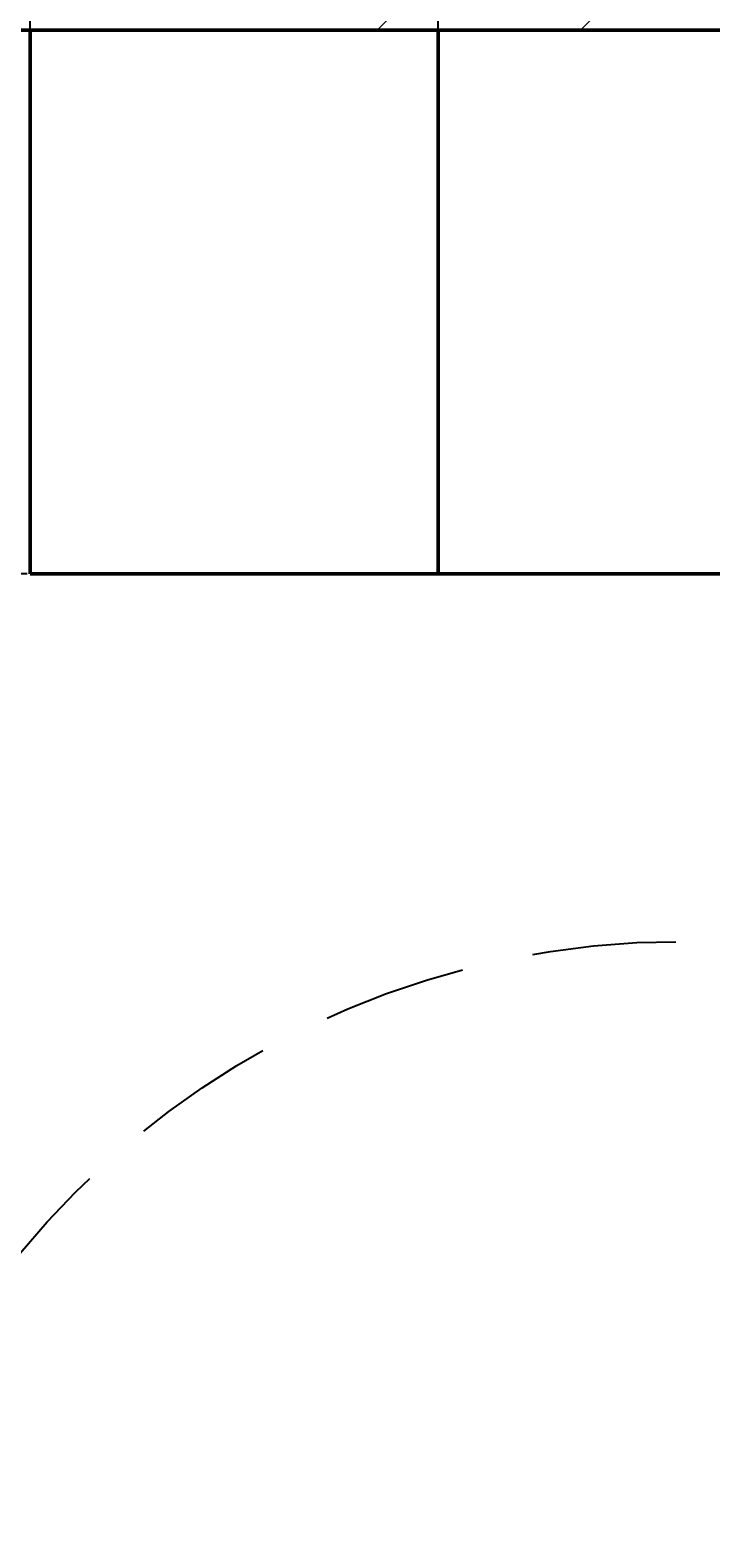
# Model space of a CAD drawing. Units: inches. Extents: x 2812 to 3051, y 1398 to 1659.
# Tile 54 of 65: x 2896 to 2911, y 1605 to 1638. Entities that reach past the tile are written whole.
import ezdxf

# ---------------------------------------------------------------- set-up
doc = ezdxf.new("R2010")
doc.units = ezdxf.units.IN
doc.linetypes.add('HIDDEN2', pattern=[4.7625, 3.175, -1.5875])
for name, color, linetype, lineweight in [('A-ANNO-DIMS', 2, 'Continuous', 18), ('S-CONC', 7, 'Continuous', 50), ('S-CONC-HIDN', 8, 'HIDDEN2', 25), ('S-CONC-PATT', 8, 'Continuous', 18)]:
    doc.layers.add(name, color=color, linetype=linetype, lineweight=lineweight)
doc.styles.get("Standard").update_dxf_attribs({"font": 'arial.ttf'})
doc.dimstyles.get("Standard").update_dxf_attribs({"dimtxt": 0.18, "dimasz": 0.18, "dimexe": 0.18, "dimexo": 0.0625, "dimgap": 0.09, "dimtad": 0, "dimtih": 1, "dimtoh": 1, "dimdec": 4, "dimzin": 0, "dimdsep": 46, "dimtxsty": 'Standard', "dimcen": 0.09, "dimadec": 0, "dimazin": 0, "dimtfac": 1, "dimtdec": 4, "dimtofl": 0, "dimtmove": 0, "dimatfit": 3, "dimfxl": 1, "dimtolj": 1, "dimtzin": 0, "dimarcsym": 0})

# ---------------------------------------------------------------- blocks, each defined once
blk = doc.blocks.new('*D18')
at = {"layer": 'A-ANNO-DIMS', "color": 0, "lineweight": -2, "transparency": 16777216}
for p, q in [((2896.385, 1625.882), (2896.385, 1659.35)), ((2905.385, 1625.882), (2905.385, 1659.35)), ((2896.565, 1659.17), (2900.736, 1659.17)), ((2905.205, 1659.17), (2901.034, 1659.17))]:
    blk.add_line(p, q, dxfattribs=at)
at = {"layer": 'A-ANNO-DIMS', "color": 0, "transparency": 16777216}
for points in [[(2896.565, 1659.2), (2896.565, 1659.14), (2896.385, 1659.17)], [(2905.205, 1659.2), (2905.205, 1659.14), (2905.385, 1659.17)]]:
    blk.add_solid(points, dxfattribs=at)
at = {"layer": 'Defpoints', "color": 0, "transparency": 16777216}
for p in [(2905.385, 1659.17), (2896.385, 1625.82), (2905.385, 1625.82)]:
    blk.add_point(p, dxfattribs=at)
at = {"layer": 'A-ANNO-DIMS', "color": 0, "transparency": 16777216, "insert": (2900.885, 1659.17), "char_height": 0.18, "attachment_point": 5}
blk.add_mtext('\\A1;9', dxfattribs=at)
blk = doc.blocks.new('*D19')
at = {"layer": 'A-ANNO-DIMS', "color": 0, "lineweight": -2, "transparency": 16777216}
for p, q in [((2905.385, 1625.882), (2905.385, 1659.35)), ((2941.385, 1625.882), (2941.385, 1659.35)), ((2905.565, 1659.17), (2923.166, 1659.17)), ((2941.205, 1659.17), (2923.604, 1659.17))]:
    blk.add_line(p, q, dxfattribs=at)
at = {"layer": 'A-ANNO-DIMS', "color": 0, "transparency": 16777216}
for points in [[(2905.565, 1659.2), (2905.565, 1659.14), (2905.385, 1659.17)], [(2941.205, 1659.2), (2941.205, 1659.14), (2941.385, 1659.17)]]:
    blk.add_solid(points, dxfattribs=at)
at = {"layer": 'Defpoints', "color": 0, "transparency": 16777216}
for p in [(2941.385, 1659.17), (2905.385, 1625.82), (2941.385, 1625.82)]:
    blk.add_point(p, dxfattribs=at)
at = {"layer": 'A-ANNO-DIMS', "color": 0, "transparency": 16777216, "insert": (2923.385, 1659.17), "char_height": 0.18, "attachment_point": 5}
blk.add_mtext('\\A1;36', dxfattribs=at)
blk = doc.blocks.new('*D38')
at = {"layer": 'A-ANNO-DIMS', "color": 0, "lineweight": -2, "transparency": 16777216}
for p, q in [((2896.322, 1625.82), (2811.806, 1625.82)), ((2811.986, 1625.64), (2811.986, 1612.5)), ((2811.986, 1599), (2811.986, 1612.14)), ((2910.679, 1598.82), (2811.806, 1598.82))]:
    blk.add_line(p, q, dxfattribs=at)
at = {"layer": 'A-ANNO-DIMS', "color": 0, "transparency": 16777216}
for points in [[(2811.956, 1625.64), (2812.016, 1625.64), (2811.986, 1625.82)], [(2811.956, 1599), (2812.016, 1599), (2811.986, 1598.82)]]:
    blk.add_solid(points, dxfattribs=at)
at = {"layer": 'Defpoints', "color": 0, "transparency": 16777216}
for p in [(2811.986, 1625.82), (2896.385, 1625.82), (2910.742, 1598.82)]:
    blk.add_point(p, dxfattribs=at)
at = {"layer": 'A-ANNO-DIMS', "color": 0, "transparency": 16777216, "insert": (2811.986, 1612.32), "char_height": 0.18, "attachment_point": 5}
blk.add_mtext('\\A1;27', dxfattribs=at)

msp = doc.modelspace()

# ---------------------------------------------------------------- hatches: boundary and pattern name
at = {"layer": 'S-CONC-PATT'}
h = msp.add_hatch(dxfattribs=at)
h.set_pattern_fill('ANSI32', color=256)
h.paths.add_polyline_path([(3027.3849, 1646.82), (2835.3849, 1646.82), (2835.3849, 1603.2296), (2844.3849, 1603.2296), (2844.3849, 1637.82), (3018.3849, 1637.82), (3018.3849, 1602.5441), (3027.3849, 1602.5441)])
h.paths.add_polyline_path([(2844.3849, 1594.2296), (2835.3849, 1594.2296), (2835.3849, 1550.82), (3027.3849, 1550.82), (3027.3849, 1593.5441), (3018.3849, 1593.5441), (3018.3849, 1559.82), (2844.3849, 1559.82)])
h.paths.add_polyline_path([(2844.3849, 1482.0354), (2835.3849, 1482.0354), (2835.3849, 1463.4959), (2844.3849, 1463.4959)])
h.paths.add_polyline_path([(2844.3849, 1461.4959), (2835.3849, 1461.4959), (2835.3849, 1416.0354), (2844.3849, 1416.0354)])
h.paths.add_polyline_path([(3027.3849, 1482.0354), (3018.3849, 1482.0354), (3018.3849, 1463.2854), (3027.3849, 1463.2854)])
h.paths.add_polyline_path([(3027.3849, 1461.2854), (3018.3849, 1461.2854), (3018.3849, 1416.0354), (3027.3849, 1416.0354)])
h.paths.add_polyline_path([(2961.3849, 1448.4738), (2952.3849, 1448.4738), (2952.3849, 1416.0354), (2961.3849, 1416.0354)])
h.paths.add_polyline_path([(2961.3849, 1462.3026), (2952.3849, 1462.3026), (2952.3849, 1450.4738), (2961.3849, 1450.4738)])
h.paths.add_polyline_path([(2961.3849, 1472.0354), (2952.3849, 1472.0354), (2952.3849, 1462.3026), (2961.3849, 1462.3026)])

# ---------------------------------------------------------------- linework, layer by layer
at = {"layer": 'S-CONC'}
for p, q in [((2844.3849, 1637.82), (3018.3849, 1637.82)), ((2896.3849, 1625.82), (2896.3849, 1637.82)), ((2914.3849, 1637.82), (2905.3849, 1637.82)), ((2905.3849, 1637.82), (2905.3849, 1625.82)), ((2896.3849, 1625.82), (2941.3849, 1625.82)), ((2905.3849, 1625.82), (2896.3849, 1625.82)), ((2905.3849, 1625.82), (2905.3849, 1625.82))]:
    msp.add_line(p, q, dxfattribs=at)
at = {"layer": 'S-CONC-HIDN'}
msp.add_circle((2910.7415, 1598.82), 18.8884, dxfattribs=at)

# ---------------------------------------------------------------- dimensions: what is measured, and where the dimension line sits
at = {"layer": 'A-ANNO-DIMS'}
for base, p1, p2, picture, middle in [((2905.3849, 1659.17), (2896.3849, 1625.82), (2905.3849, 1625.82), '*D18', (2900.8849, 1659.17)), ((2941.3849, 1659.17), (2905.3849, 1625.82), (2941.3849, 1625.82), '*D19', (2923.3849, 1659.17))]:
    dim = msp.add_linear_dim(base=base, p1=p1, p2=p2, dimstyle='Standard', override={"dimdec": 0, "dimlfac": 1, "dimrnd": 0, "dimzin": 0, "dimdsep": 46, "dimlunit": 2}, dxfattribs=at)
    dim.commit()
    dim.dimension.update_dxf_attribs({"geometry": picture, "text_midpoint": middle})
dim = msp.add_linear_dim(base=(2811.9855, 1625.82), p1=(2910.7415, 1598.82), p2=(2896.3849, 1625.82), angle=90, dimstyle='Standard', override={"dimdec": 0, "dimlfac": 1, "dimrnd": 0, "dimzin": 0, "dimdsep": 46, "dimlunit": 2}, dxfattribs=at)
dim.commit()
dim.dimension.update_dxf_attribs({"geometry": '*D38', "text_midpoint": (2811.9855, 1612.32)})

doc.saveas('drawing.dxf')
